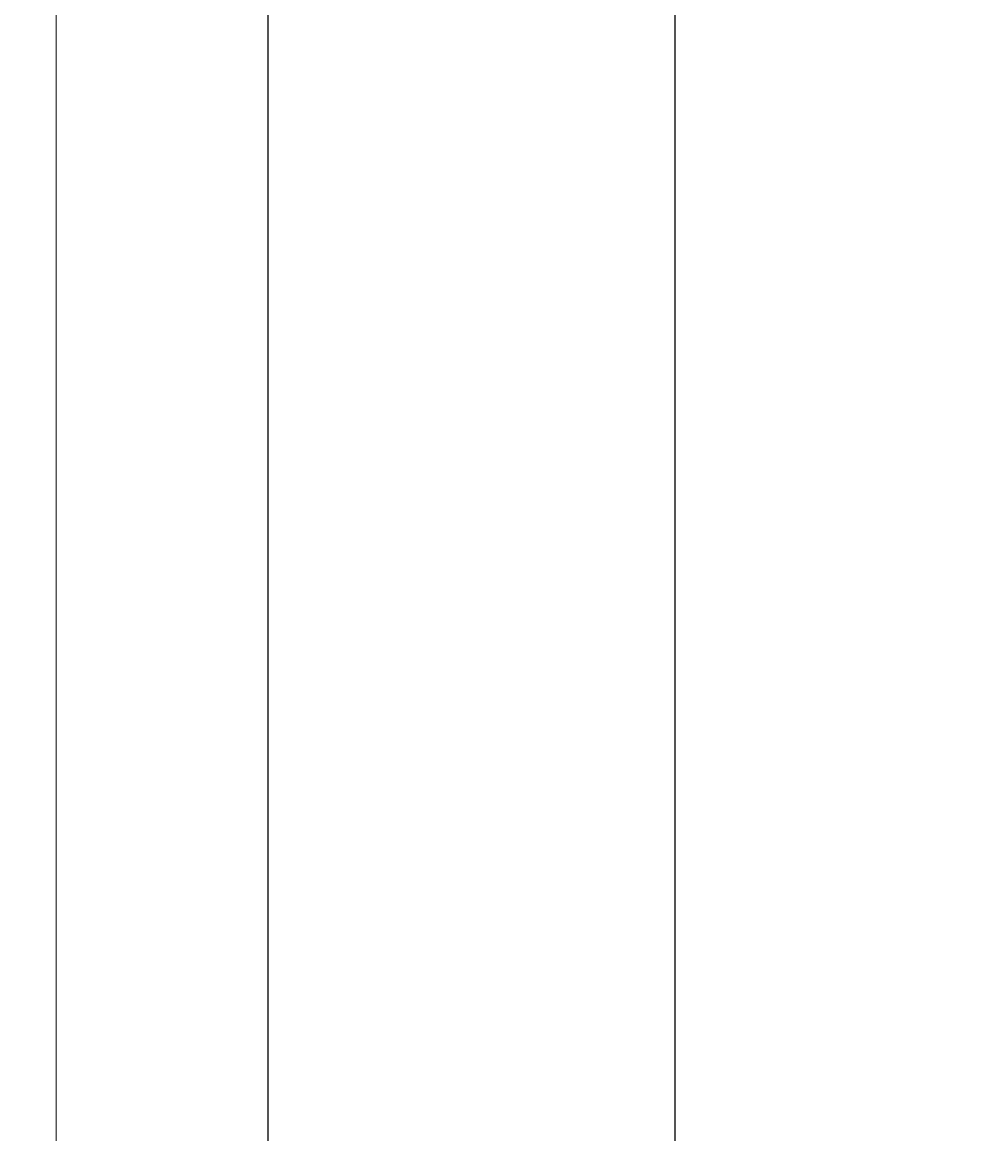
# Model space of a CAD drawing. Units: inches. Extents: x -46 to 1145, y -527 to 760.
# Tile 8 of 57: x 187 to 272, y -270 to -172. Entities that reach past the tile are written whole.
import ezdxf

# ---------------------------------------------------------------- set-up
doc = ezdxf.new("R2010")
doc.units = ezdxf.units.IN
doc.header["$MEASUREMENT"] = 0
doc.layers.add('A-ANNO-DIMS', color=2, linetype='Continuous', lineweight=18)
doc.layers.add('C-ROAD', color=9, linetype='Continuous', lineweight=18)
doc.styles.get("Standard").update_dxf_attribs({"font": 'arial.ttf'})
doc.dimstyles.get("Standard").update_dxf_attribs({"dimtxt": 0.18, "dimasz": 0.18, "dimexe": 0.18, "dimexo": 0.0625, "dimgap": 0.09, "dimtad": 0, "dimtih": 1, "dimtoh": 1, "dimdec": 0, "dimzin": 0, "dimdsep": 46, "dimlunit": 3, "dimtxsty": 'Standard', "dimcen": 0.09, "dimadec": 0, "dimazin": 0, "dimtfac": 1, "dimtdec": 0, "dimtofl": 0, "dimtmove": 0, "dimatfit": 3, "dimfxl": 1, "dimtolj": 1, "dimtzin": 0, "dimarcsym": 0})

# ---------------------------------------------------------------- blocks, each defined once
blk = doc.blocks.new('*D695')
at = {"layer": 'A-ANNO-DIMS', "color": 0, "lineweight": -2, "transparency": 16777216}
for p, q in [((208.273, 221.455), (208.273, -527.262)), ((244.273, 221.455), (244.273, -527.262)), ((208.453, -527.082), (226.054, -527.082)), ((244.093, -527.082), (226.492, -527.082))]:
    blk.add_line(p, q, dxfattribs=at)
at = {"layer": 'A-ANNO-DIMS', "color": 0, "transparency": 16777216}
for points in [[(208.453, -527.052), (208.453, -527.112), (208.273, -527.082)], [(244.093, -527.052), (244.093, -527.112), (244.273, -527.082)]]:
    blk.add_solid(points, dxfattribs=at)
at = {"layer": 'Defpoints', "color": 0, "transparency": 16777216}
for p in [(208.273, 221.518), (244.273, 221.518), (244.273, -527.082)]:
    blk.add_point(p, dxfattribs=at)
at = {"layer": 'A-ANNO-DIMS', "color": 0, "transparency": 16777216, "insert": (226.273, -527.082), "char_height": 0.18, "attachment_point": 5}
blk.add_mtext('\\A1;36', dxfattribs=at)
blk = doc.blocks.new('*D702')
at = {"layer": 'A-ANNO-DIMS', "color": 0, "lineweight": -2, "transparency": 16777216}
for p, q in [((189.626, -39.482), (1145.344, -39.482)), ((1145.164, -39.662), (1145.164, -249.301)), ((1145.164, -459.302), (1145.164, -249.664)), ((183.626, -459.482), (1145.344, -459.482))]:
    blk.add_line(p, q, dxfattribs=at)
at = {"layer": 'A-ANNO-DIMS', "color": 0, "transparency": 16777216}
for points in [[(1145.134, -39.662), (1145.194, -39.662), (1145.164, -39.482)], [(1145.134, -459.302), (1145.194, -459.302), (1145.164, -459.482)]]:
    blk.add_solid(points, dxfattribs=at)
at = {"layer": 'Defpoints', "color": 0, "transparency": 16777216}
for p in [(189.564, -39.482), (1145.164, -39.482), (183.564, -459.482)]:
    blk.add_point(p, dxfattribs=at)
at = {"layer": 'A-ANNO-DIMS', "color": 0, "transparency": 16777216, "insert": (1145.164, -249.482), "char_height": 0.18, "attachment_point": 5}
blk.add_mtext('\\A1;420', dxfattribs=at)

msp = doc.modelspace()

# ---------------------------------------------------------------- linework, layer by layer
at = {"layer": 'C-ROAD'}
msp.add_line((189.5637, 221.5176), (189.5637, -468.4824), dxfattribs=at)

# ---------------------------------------------------------------- dimensions: what is measured, and where the dimension line sits
at = {"layer": 'A-ANNO-DIMS'}
dim = msp.add_linear_dim(base=(244.2731, -527.0824), p1=(208.2731, 221.5176), p2=(244.2731, 221.5176), dimstyle='Standard', override={"dimdec": 0, "dimlfac": 1, "dimrnd": 0, "dimzin": 0, "dimdsep": 46, "dimlunit": 2}, dxfattribs=at)
dim.commit()
dim.dimension.update_dxf_attribs({"geometry": '*D695', "text_midpoint": (226.2731, -527.0824)})
dim = msp.add_linear_dim(base=(1145.1637, -39.4824), p1=(183.5637, -459.4824), p2=(189.5637, -39.4824), angle=90, dimstyle='Standard', override={"dimdec": 0, "dimlfac": 1, "dimrnd": 0, "dimzin": 0, "dimdsep": 46, "dimlunit": 2}, dxfattribs=at)
dim.commit()
dim.dimension.update_dxf_attribs({"geometry": '*D702', "text_midpoint": (1145.1637, -249.4824)})

doc.saveas('drawing.dxf')
